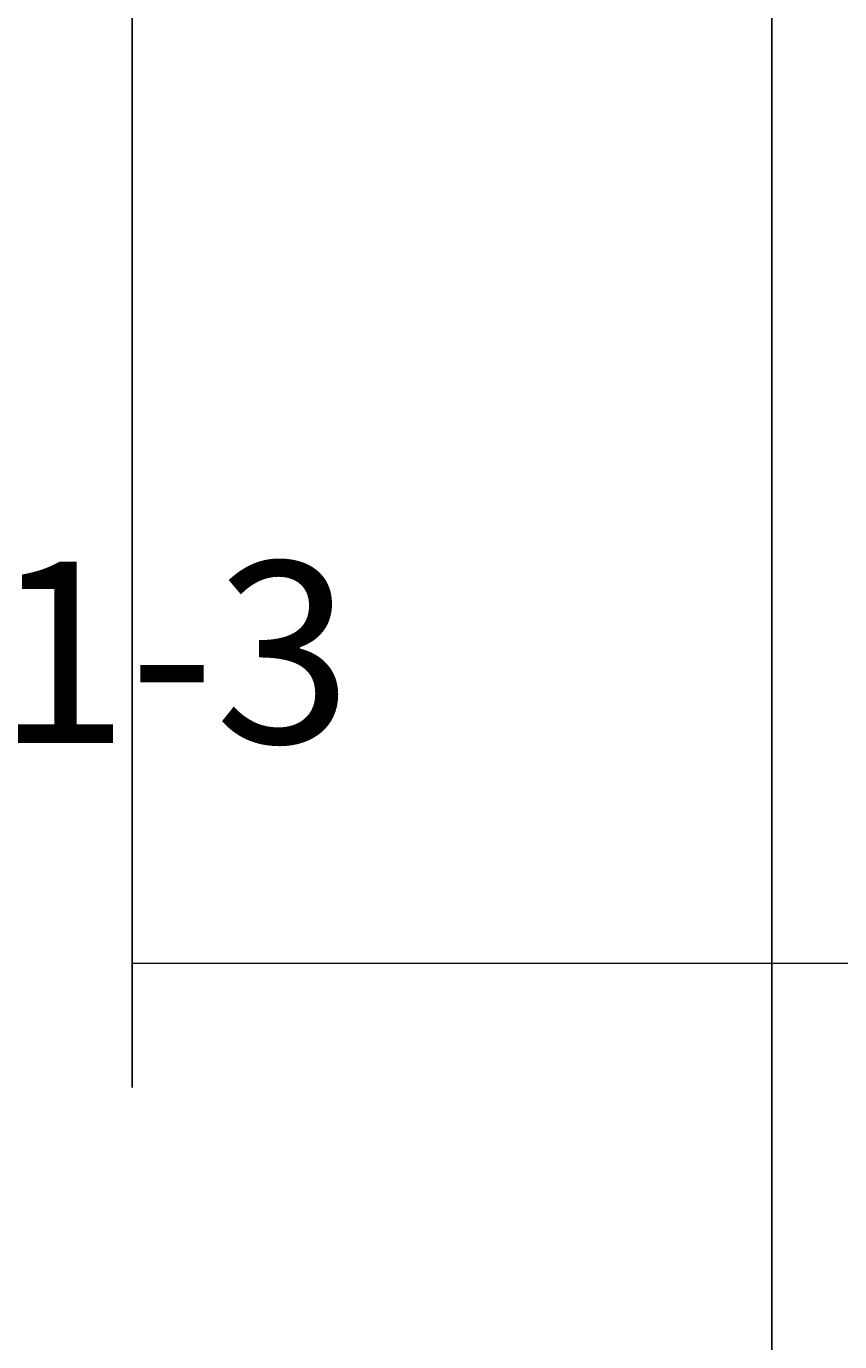
# Model space of a CAD drawing. Units: inches. Extents: x 738 to 1068, y 378 to 757.
# Tile 10 of 41: x 806 to 833, y 449 to 492. Entities that reach past the tile are written whole.
import ezdxf

# ---------------------------------------------------------------- set-up
doc = ezdxf.new("R2010")
doc.units = ezdxf.units.IN
doc.header["$MEASUREMENT"] = 0
for name, color, linetype, lineweight in [('A-ANNO-DIMS', 2, 'Continuous', 18), ('E-ANNO-TEXT', 7, 'Continuous', 18), ('E-CTRL-CONT', 4, 'Continuous', 25), ('E-CTRL-WIRE', 7, 'Continuous', 18)]:
    doc.layers.add(name, color=color, linetype=linetype, lineweight=lineweight)
doc.styles.get("Standard").update_dxf_attribs({"font": 'arial.ttf'})
doc.dimstyles.get("Standard").update_dxf_attribs({"dimtxt": 0.18, "dimasz": 0.18, "dimexe": 0.18, "dimexo": 0.0625, "dimgap": 0.09, "dimtad": 0, "dimtih": 1, "dimtoh": 1, "dimdec": 4, "dimzin": 0, "dimdsep": 46, "dimtxsty": 'Standard', "dimcen": 0.09, "dimadec": 0, "dimazin": 0, "dimtfac": 1, "dimtdec": 4, "dimtofl": 0, "dimtmove": 0, "dimatfit": 3, "dimfxl": 1, "dimtolj": 1, "dimtzin": 0, "dimarcsym": 0})

# ---------------------------------------------------------------- blocks, each defined once
blk = doc.blocks.new('CR-AUX-CONTACT-NO')
for p, q in [((0, 8.72), (0, 0)), ((8.265, 8.72), (8.265, 0))]:
    blk.add_line(p, q)
blk = doc.blocks.new('*D32')
at = {"layer": 'A-ANNO-DIMS', "color": 0, "lineweight": -2, "transparency": 16777216}
for p, q in [((809.38, 461.454), (809.38, 756.505)), ((809.56, 756.325), (822.41, 756.325)), ((836.052, 756.325), (823.202, 756.325)), ((836.232, 461.277), (836.232, 756.505))]:
    blk.add_line(p, q, dxfattribs=at)
at = {"layer": 'A-ANNO-DIMS', "color": 0, "transparency": 16777216}
for points in [[(809.56, 756.355), (809.56, 756.295), (809.38, 756.325)], [(836.052, 756.355), (836.052, 756.295), (836.232, 756.325)]]:
    blk.add_solid(points, dxfattribs=at)
at = {"layer": 'Defpoints', "color": 0, "transparency": 16777216}
for p in [(836.232, 756.325), (809.38, 461.392), (836.232, 461.214)]:
    blk.add_point(p, dxfattribs=at)
at = {"layer": 'A-ANNO-DIMS', "color": 0, "transparency": 16777216, "insert": (822.806, 756.325), "char_height": 0.18, "attachment_point": 5}
blk.add_mtext('\\A1;26.85', dxfattribs=at)
blk = doc.blocks.new('*D34')
at = {"layer": 'A-ANNO-DIMS', "color": 0, "lineweight": -2, "transparency": 16777216}
for p, q in [((781.49, 686.266), (781.49, 378.239)), ((830.489, 686.266), (830.489, 378.239)), ((781.67, 378.419), (805.767, 378.419)), ((830.309, 378.419), (806.212, 378.419))]:
    blk.add_line(p, q, dxfattribs=at)
at = {"layer": 'A-ANNO-DIMS', "color": 0, "transparency": 16777216}
for points in [[(781.67, 378.449), (781.67, 378.389), (781.49, 378.419)], [(830.309, 378.449), (830.309, 378.389), (830.489, 378.419)]]:
    blk.add_solid(points, dxfattribs=at)
at = {"layer": 'Defpoints', "color": 0, "transparency": 16777216}
for p in [(781.49, 686.329), (830.489, 686.329), (830.489, 378.419)]:
    blk.add_point(p, dxfattribs=at)
at = {"layer": 'A-ANNO-DIMS', "color": 0, "transparency": 16777216, "insert": (805.99, 378.419), "char_height": 0.18, "attachment_point": 5}
blk.add_mtext('\\A1;49', dxfattribs=at)
blk = doc.blocks.new('*D38')
at = {"layer": 'A-ANNO-DIMS', "color": 0, "lineweight": -2, "transparency": 16777216}
for p, q in [((781.485, 593.017), (781.485, 378.239)), ((887.04, 593.067), (887.04, 378.239)), ((781.665, 378.419), (833.807, 378.419)), ((886.86, 378.419), (834.718, 378.419))]:
    blk.add_line(p, q, dxfattribs=at)
at = {"layer": 'A-ANNO-DIMS', "color": 0, "transparency": 16777216}
for points in [[(781.665, 378.449), (781.665, 378.389), (781.485, 378.419)], [(886.86, 378.449), (886.86, 378.389), (887.04, 378.419)]]:
    blk.add_solid(points, dxfattribs=at)
at = {"layer": 'Defpoints', "color": 0, "transparency": 16777216}
for p in [(887.04, 593.13), (781.485, 593.08), (887.04, 378.419)]:
    blk.add_point(p, dxfattribs=at)
at = {"layer": 'A-ANNO-DIMS', "color": 0, "transparency": 16777216, "insert": (834.263, 378.419), "char_height": 0.18, "attachment_point": 5}
blk.add_mtext('\\A1;105.56', dxfattribs=at)

msp = doc.modelspace()

# ---------------------------------------------------------------- linework, layer by layer
at = {"layer": 'E-CTRL-WIRE'}
msp.add_line((809.3803, 461.3919), (865.0964, 461.3919), dxfattribs=at)

# ---------------------------------------------------------------- block references
at = {"layer": 'E-CTRL-CONT'}
msp.add_blockref('CR-AUX-CONTACT-NO', (801.115, 457.29), dxfattribs=at)

# ---------------------------------------------------------------- texts
at = {"layer": 'E-ANNO-TEXT'}
msp.add_text('CR1-3', height=5.97842, dxfattribs=at).set_placement((794.3655, 468.6537))

# ---------------------------------------------------------------- dimensions: what is measured, and where the dimension line sits
at = {"layer": 'A-ANNO-DIMS'}
for base, p1, p2, override, picture, middle in [((836.2324, 756.3251), (809.3803, 461.3919), (836.2324, 461.214), {"dimdec": 2, "dimlfac": 1, "dimrnd": 0, "dimzin": 0, "dimdsep": 46, "dimlunit": 2}, '*D32', (822.8064, 756.3251)), ((830.4893, 378.4191), (781.4897, 686.329), (830.4893, 686.329), {"dimdec": 0, "dimlfac": 1, "dimrnd": 0, "dimzin": 0, "dimdsep": 46, "dimlunit": 2}, '*D34', (805.9895, 378.4191)), ((887.0404, 378.4191), (781.4846, 593.0796), (887.0404, 593.1296), {"dimdec": 2, "dimlfac": 1, "dimrnd": 0, "dimzin": 0, "dimdsep": 46, "dimlunit": 2}, '*D38', (834.2625, 378.4191))]:
    dim = msp.add_linear_dim(base=base, p1=p1, p2=p2, dimstyle='Standard', override=override, dxfattribs=at)
    dim.commit()
    dim.dimension.update_dxf_attribs({"geometry": picture, "text_midpoint": middle})

doc.saveas('drawing.dxf')
